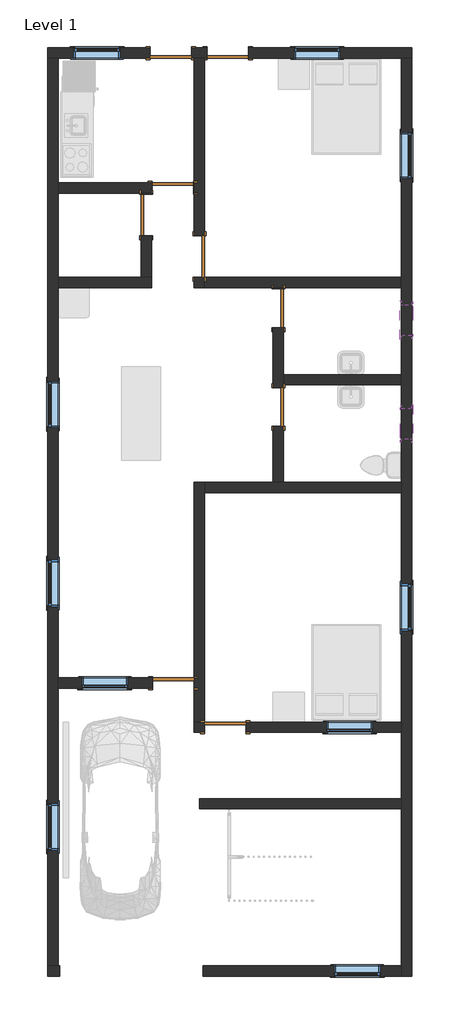
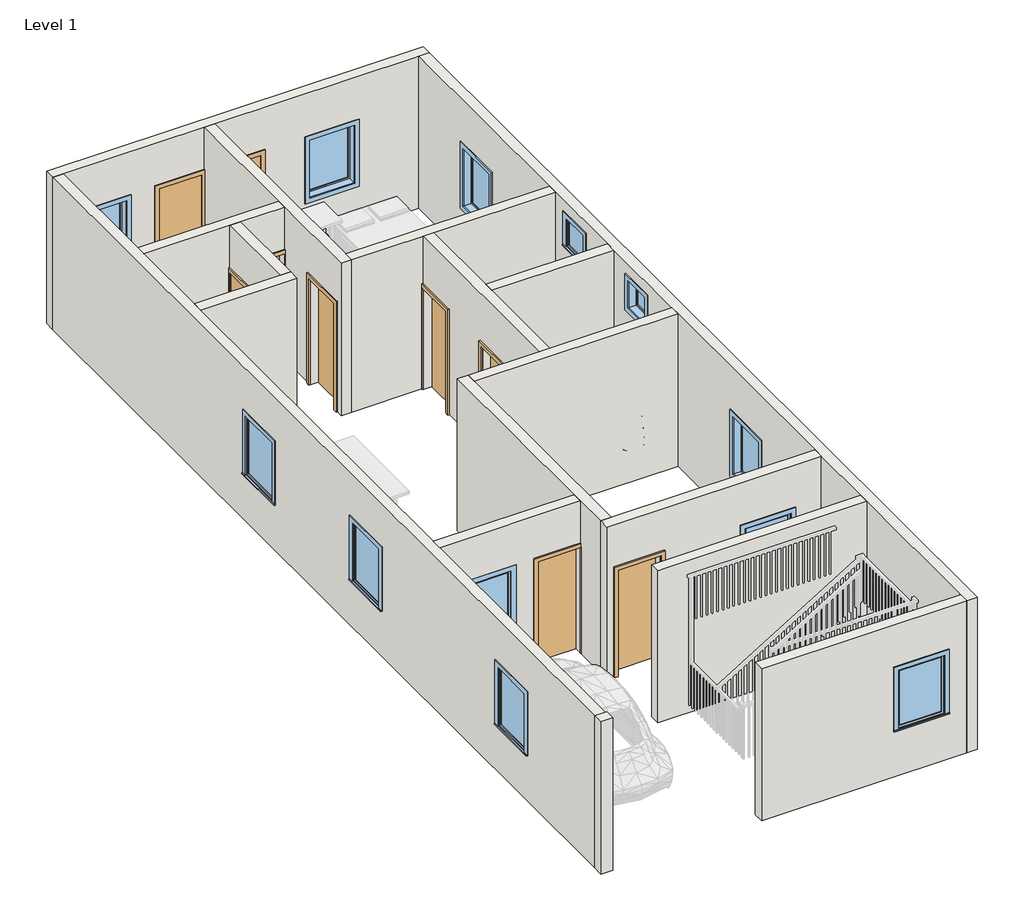
# One storey, part 1 of 3: 17 walls, 12 windows, 9 doors.
"""IFC4 building model written with IfcOpenShell, lengths in millimetres."""

from ifc_helpers import new_model, si_unit, frame, origin, origin_with_axes, place, context, project, spatial, polyline, outline, extrude, faceted_brep, transform, mapped, element, save
from components import door_53b1b562, door_64d5ae29, door_0d629d65, window_8a4441b2, window_bec2521a, window_e41d21a6

model = new_model("IFC4")

# Units and contexts
model_context = context("Model", 3, world=origin())
ifc_project = project(units=[si_unit("LENGTHUNIT", "METRE", prefix="MILLI")], contexts=[model_context])

# Site, building, storey
site = spatial("IfcSite", under=ifc_project)
building = spatial("IfcBuilding", under=site)
storey = spatial("IfcBuildingStorey", under=building, Name="Level 1", Elevation=0.0)

# Doors
placement = place(None, origin())
door_shape = door_53b1b562(model_context)
element("IfcDoor", 1, ObjectType="Single-Flush : 30\" x 80\"", at=placement, inside=storey, context=model_context, shape_type="MappedRepresentation", body=[
    mapped(door_shape, transform((-5398.5370113, 5721.2865244, 0.0), x_axis=(0.0, 1.0, 0.0), y_axis=(-1.0, 0.0, 0.0), z_axis=(0.0, 0.0, 1.0))),
])
element("IfcDoor", 2, ObjectType="Single-Flush : 30\" x 80\"", at=placement, inside=storey, context=model_context, shape_type="MappedRepresentation", body=[
    mapped(door_shape, transform((-5398.5370113, 3790.8865244, 0.0), x_axis=(0.0, 1.0, 0.0), y_axis=(-1.0, 0.0, 0.0), z_axis=(0.0, 0.0, 1.0))),
])
door_2_shape = door_64d5ae29(model_context)
element("IfcDoor", 3, ObjectType="Single-Flush : 32\" x 84\"", at=placement, inside=storey, context=model_context, shape_type="MappedRepresentation", body=[
    mapped(door_2_shape, transform((-7468.6370113, 8083.4865244, 0.0), x_axis=(1.0, 0.0, 0.0), y_axis=(0.0, 1.0, 0.0), z_axis=(0.0, 0.0, 1.0))),
])
element("IfcDoor", 4, ObjectType="Single-Flush : 32\" x 84\"", at=placement, inside=storey, context=model_context, shape_type="MappedRepresentation", body=[
    mapped(door_2_shape, transform((-7989.3370113, 7550.0865244, 0.0), x_axis=(0.0, 1.0, 0.0), y_axis=(-1.0, 0.0, 0.0), z_axis=(0.0, 0.0, 1.0))),
])
element("IfcDoor", 5, ObjectType="Single-Flush : 32\" x 84\"", at=placement, inside=storey, context=model_context, shape_type="MappedRepresentation", body=[
    mapped(door_2_shape, transform((-6947.9370113, 6737.2865244, 0.0), x_axis=(0.0, -1.0, 0.0), y_axis=(1.0, 0.0, 0.0), z_axis=(0.0, 0.0, 1.0))),
])
element("IfcDoor", 6, ObjectType="Single-Flush : 32\" x 84\"", at=placement, inside=storey, context=model_context, shape_type="MappedRepresentation", body=[
    mapped(door_2_shape, transform((-6389.1370113, 10725.0865244, 0.0), x_axis=(-1.0, 0.0, 0.0), y_axis=(0.0, -1.0, 0.0), z_axis=(0.0, 0.0, 1.0))),
])
element("IfcDoor", 7, ObjectType="Single-Flush : 32\" x 84\"", at=placement, inside=storey, context=model_context, shape_type="MappedRepresentation", body=[
    mapped(door_2_shape, transform((-7455.9370113, -1619.3134756, 0.0), x_axis=(1.0, 0.0, 0.0), y_axis=(0.0, 1.0, 0.0), z_axis=(0.0, 0.0, 1.0))),
])
door_3_shape = door_0d629d65(model_context)
element("IfcDoor", 8, ObjectType="Single-Flush : 32\" x 84\"", at=placement, inside=storey, context=model_context, shape_type="MappedRepresentation", body=[
    mapped(door_3_shape, transform((-7506.7370113, 10725.0865244, 0.0), x_axis=(1.0, 0.0, 0.0), y_axis=(0.0, 1.0, 0.0), z_axis=(0.0, 0.0, 1.0))),
])
element("IfcDoor", 9, ObjectType="Single-Flush : 32\" x 84\"", at=placement, inside=storey, context=model_context, shape_type="MappedRepresentation", body=[
    mapped(door_3_shape, transform((-6439.9370113, -2482.9134756, 0.0), x_axis=(-1.0, 0.0, 0.0), y_axis=(0.0, -1.0, 0.0), z_axis=(0.0, 0.0, 1.0))),
])

# Walls
element("IfcWall", 10, ObjectType="Generic - 8\"", at=placement, inside=storey, context=model_context, shape_type="Brep", body=[
    faceted_brep([(-7100.3370113, 10623.4865244, 0.0), (-7049.5370113, 10623.4865244, 0.0), (-6846.3370113, 10623.4865244, 0.0), (-6795.5370113, 10623.4865244, 0.0), (-6795.5370113, 10623.4865244, 2133.6), (-5982.7370113, 10623.4865244, 2133.6), (-5982.7370113, 10623.4865244, 0.0), (-2985.5370113, 10623.4865244, 0.0), (-2782.3370113, 10623.4865244, 0.0), (-2782.3370113, 10623.4865244, 3048.0), (-2985.5370113, 10623.4865244, 3048.0), (-6846.3370113, 10623.4865244, 3048.0), (-7049.5370113, 10623.4865244, 3048.0), (-9716.5370113, 10623.4865244, 3048.0), (-9919.7370113, 10623.4865244, 3048.0), (-9919.7370113, 10623.4865244, 0.0), (-9716.5370113, 10623.4865244, 0.0), (-7913.1370113, 10623.4865244, 0.0), (-7913.1370113, 10623.4865244, 2133.6), (-7100.3370113, 10623.4865244, 2133.6), (-4179.3370113, 10623.4865244, 2133.6), (-4179.3370113, 10623.4865244, 914.4), (-5093.7370113, 10623.4865244, 914.4), (-5093.7370113, 10623.4865244, 2133.6), (-8497.3370113, 10623.4865244, 2133.6), (-8497.3370113, 10623.4865244, 914.4), (-9411.7370113, 10623.4865244, 914.4), (-9411.7370113, 10623.4865244, 2133.6), (-6795.5370113, 10826.6865244, 2133.6), (-6795.5370113, 10826.6865244, 0.0), (-7100.3370113, 10826.6865244, 0.0), (-7100.3370113, 10826.6865244, 2133.6), (-7913.1370113, 10826.6865244, 2133.6), (-7913.1370113, 10826.6865244, 0.0), (-9919.7370113, 10826.6865244, 0.0), (-9919.7370113, 10826.6865244, 3048.0), (-2782.3370113, 10826.6865244, 3048.0), (-2782.3370113, 10826.6865244, 0.0), (-5982.7370113, 10826.6865244, 0.0), (-5982.7370113, 10826.6865244, 2133.6), (-4179.3370113, 10826.6865244, 2133.6), (-5093.7370113, 10826.6865244, 2133.6), (-5093.7370113, 10826.6865244, 914.4), (-4179.3370113, 10826.6865244, 914.4), (-8497.3370113, 10826.6865244, 2133.6), (-9411.7370113, 10826.6865244, 2133.6), (-9411.7370113, 10826.6865244, 914.4), (-8497.3370113, 10826.6865244, 914.4)], [[[0, 1, 2, 3, 4, 5, 6, 7, 8, 9, 10, 11, 12, 13, 14, 15, 16, 17, 18, 19], [20, 21, 22, 23], [24, 25, 26, 27]], [[28, 29, 30, 31, 32, 33, 34, 35, 36, 37, 38, 39], [40, 41, 42, 43], [44, 45, 46, 47]], [[17, 16, 15, 34, 33]], [[38, 37, 8, 7, 6]], [[30, 29, 3, 2, 1, 0]], [[14, 13, 12, 11, 10, 9, 36, 35]], [[9, 8, 37, 36]], [[15, 14, 35, 34]], [[31, 30, 0, 19]], [[32, 31, 19, 18]], [[33, 32, 18, 17]], [[4, 3, 29, 28]], [[5, 4, 28, 39]], [[6, 5, 39, 38]], [[21, 20, 40, 43]], [[22, 21, 43, 42]], [[23, 22, 42, 41]], [[20, 23, 41, 40]], [[25, 24, 44, 47]], [[26, 25, 47, 46]], [[27, 26, 46, 45]], [[24, 27, 45, 44]]]),
])
element("IfcWall", 11, ObjectType="Generic - 8\"", at=placement, inside=storey, context=model_context, shape_type="Brep", body=[
    faceted_brep([(-2985.5370113, 10623.4865244, 0.0), (-2985.5370113, 6330.8865244, 0.0), (-2985.5370113, 6127.6865244, 0.0), (-2985.5370113, 4425.8865244, 0.0), (-2985.5370113, 4222.6865244, 0.0), (-2985.5370113, 2317.6865244, 0.0), (-2985.5370113, 2114.4865244, 0.0), (-2985.5370113, -2381.3134756, 0.0), (-2985.5370113, -2584.5134756, 0.0), (-2985.5370113, -3879.9134756, 0.0), (-2985.5370113, -4083.1134756, 0.0), (-2985.5370113, -7156.5134756, 0.0), (-2985.5370113, -7359.7134756, 0.0), (-2985.5370113, -7359.7134756, 3048.0), (-2985.5370113, -7156.5134756, 3048.0), (-2985.5370113, -4083.1134756, 3048.0), (-2985.5370113, -3879.9134756, 3048.0), (-2985.5370113, -2584.5134756, 3048.0), (-2985.5370113, -2381.3134756, 3048.0), (-2985.5370113, 2114.4865244, 3048.0), (-2985.5370113, 2317.6865244, 3048.0), (-2985.5370113, 4222.6865244, 3048.0), (-2985.5370113, 4425.8865244, 3048.0), (-2985.5370113, 6127.6865244, 3048.0), (-2985.5370113, 6330.8865244, 3048.0), (-2985.5370113, 10623.4865244, 3048.0), (-2985.5370113, -590.6134756, 2133.6), (-2985.5370113, -590.6134756, 914.4), (-2985.5370113, 323.7865244, 914.4), (-2985.5370113, 323.7865244, 2133.6), (-2985.5370113, 8261.2865244, 2133.6), (-2985.5370113, 8261.2865244, 914.4), (-2985.5370113, 9175.6865244, 914.4), (-2985.5370113, 9175.6865244, 2133.6), (-2985.5370113, 5797.4865244, 2768.6), (-2985.5370113, 5187.8865244, 2768.6), (-2985.5370113, 5187.8865244, 2159.0), (-2985.5370113, 5797.4865244, 2159.0), (-2985.5370113, 3155.8865244, 2768.6), (-2985.5370113, 3155.8865244, 2159.0), (-2985.5370113, 3765.4865244, 2159.0), (-2985.5370113, 3765.4865244, 2768.6), (-2782.3370113, 10623.4865244, 0.0), (-2782.3370113, 10623.4865244, 3048.0), (-2782.3370113, -7359.7134756, 3048.0), (-2782.3370113, -7359.7134756, 0.0), (-2782.3370113, -590.6134756, 2133.6), (-2782.3370113, 323.7865244, 2133.6), (-2782.3370113, 323.7865244, 914.4), (-2782.3370113, -590.6134756, 914.4), (-2782.3370113, 8261.2865244, 2133.6), (-2782.3370113, 9175.6865244, 2133.6), (-2782.3370113, 9175.6865244, 914.4), (-2782.3370113, 8261.2865244, 914.4), (-2782.3370113, 5797.4865244, 2768.6), (-2782.3370113, 5797.4865244, 2159.0), (-2782.3370113, 5187.8865244, 2159.0), (-2782.3370113, 5187.8865244, 2768.6), (-2782.3370113, 3155.8865244, 2768.6), (-2782.3370113, 3765.4865244, 2768.6), (-2782.3370113, 3765.4865244, 2159.0), (-2782.3370113, 3155.8865244, 2159.0)], [[[0, 1, 2, 3, 4, 5, 6, 7, 8, 9, 10, 11, 12, 13, 14, 15, 16, 17, 18, 19, 20, 21, 22, 23, 24, 25], [26, 27, 28, 29], [30, 31, 32, 33], [34, 35, 36, 37], [38, 39, 40, 41]], [[42, 43, 44, 45], [46, 47, 48, 49], [50, 51, 52, 53], [54, 55, 56, 57], [58, 59, 60, 61]], [[12, 11, 10, 9, 8, 7, 6, 5, 4, 3, 2, 1, 0, 42, 45]], [[25, 24, 23, 22, 21, 20, 19, 18, 17, 16, 15, 14, 13, 44, 43]], [[0, 25, 43, 42]], [[13, 12, 45, 44]], [[27, 26, 46, 49]], [[28, 27, 49, 48]], [[29, 28, 48, 47]], [[26, 29, 47, 46]], [[31, 30, 50, 53]], [[32, 31, 53, 52]], [[33, 32, 52, 51]], [[30, 33, 51, 50]], [[55, 54, 34, 37]], [[56, 55, 37, 36]], [[57, 56, 36, 35]], [[54, 57, 35, 34]], [[39, 38, 58, 61]], [[40, 39, 61, 60]], [[41, 40, 60, 59]], [[38, 41, 59, 58]]]),
])
element("IfcWall", 12, ObjectType="Generic - 8\"", at=placement, inside=storey, context=model_context, shape_type="SweptSolid", body=[
    extrude(outline(polyline([(0.0, -2985.5370113), (3048.0, -2985.5370113), (3048.0, -6871.7370113), (0.0, -6871.7370113), (0.0, -2985.5370113)]), holes=[polyline([(2133.6, -4306.3370113), (2133.6, -3391.9370113), (914.4, -3391.9370113), (914.4, -4306.3370113), (2133.6, -4306.3370113)])]), frame((0.0, -7359.7134756, 0.0), z_axis=(0.0, 1.0, 0.0), x_axis=(0.0, 0.0, 1.0)), (0.0, 0.0, 1.0), 203.2),
])
element("IfcWall", 13, ObjectType="Generic - 8\"", at=placement, inside=storey, context=model_context, shape_type="Brep", body=[
    faceted_brep([(-9716.5370113, -7156.5134756, 0.0), (-9716.5370113, -1720.9134756, 0.0), (-9716.5370113, -1517.7134756, 0.0), (-9716.5370113, 6127.6865244, 0.0), (-9716.5370113, 6330.8865244, 0.0), (-9716.5370113, 7981.8865244, 0.0), (-9716.5370113, 8185.0865244, 0.0), (-9716.5370113, 10623.4865244, 0.0), (-9716.5370113, 10623.4865244, 3048.0), (-9716.5370113, 8185.0865244, 3048.0), (-9716.5370113, 7981.8865244, 3048.0), (-9716.5370113, 6330.8865244, 3048.0), (-9716.5370113, 6127.6865244, 3048.0), (-9716.5370113, -1517.7134756, 3048.0), (-9716.5370113, -1720.9134756, 3048.0), (-9716.5370113, -7156.5134756, 3048.0), (-9716.5370113, 4298.8865244, 2133.6), (-9716.5370113, 4298.8865244, 914.4), (-9716.5370113, 3384.4865244, 914.4), (-9716.5370113, 3384.4865244, 2133.6), (-9716.5370113, 793.6865244, 2133.6), (-9716.5370113, 793.6865244, 914.4), (-9716.5370113, -120.7134756, 914.4), (-9716.5370113, -120.7134756, 2133.6), (-9716.5370113, -3981.5134756, 2133.6), (-9716.5370113, -3981.5134756, 914.4), (-9716.5370113, -4895.9134756, 914.4), (-9716.5370113, -4895.9134756, 2133.6), (-9919.7370113, -7156.5134756, 0.0), (-9919.7370113, -7156.5134756, 3048.0), (-9919.7370113, 10623.4865244, 3048.0), (-9919.7370113, 10623.4865244, 0.0), (-9919.7370113, 4298.8865244, 2133.6), (-9919.7370113, 3384.4865244, 2133.6), (-9919.7370113, 3384.4865244, 914.4), (-9919.7370113, 4298.8865244, 914.4), (-9919.7370113, 793.6865244, 2133.6), (-9919.7370113, -120.7134756, 2133.6), (-9919.7370113, -120.7134756, 914.4), (-9919.7370113, 793.6865244, 914.4), (-9919.7370113, -3981.5134756, 2133.6), (-9919.7370113, -4895.9134756, 2133.6), (-9919.7370113, -4895.9134756, 914.4), (-9919.7370113, -3981.5134756, 914.4)], [[[0, 1, 2, 3, 4, 5, 6, 7, 8, 9, 10, 11, 12, 13, 14, 15], [16, 17, 18, 19], [20, 21, 22, 23], [24, 25, 26, 27]], [[28, 29, 30, 31], [32, 33, 34, 35], [36, 37, 38, 39], [40, 41, 42, 43]], [[7, 6, 5, 4, 3, 2, 1, 0, 28, 31]], [[15, 14, 13, 12, 11, 10, 9, 8, 30, 29]], [[8, 7, 31, 30]], [[0, 15, 29, 28]], [[17, 16, 32, 35]], [[18, 17, 35, 34]], [[19, 18, 34, 33]], [[16, 19, 33, 32]], [[21, 20, 36, 39]], [[22, 21, 39, 38]], [[23, 22, 38, 37]], [[20, 23, 37, 36]], [[25, 24, 40, 43]], [[26, 25, 43, 42]], [[27, 26, 42, 41]], [[24, 27, 41, 40]]]),
])
element("IfcWall", 14, ObjectType="Generic - 8\"", at=placement, inside=storey, context=model_context, shape_type="Brep", body=[
    faceted_brep([(-7062.2370113, 7981.8865244, 2133.6), (-7062.2370113, 7981.8865244, 0.0), (-7049.5370113, 7981.8865244, 0.0), (-7049.5370113, 7981.8865244, 3048.0), (-7887.7370113, 7981.8865244, 3048.0), (-8090.9370113, 7981.8865244, 3048.0), (-9716.5370113, 7981.8865244, 3048.0), (-9716.5370113, 7981.8865244, 0.0), (-8090.9370113, 7981.8865244, 0.0), (-7887.7370113, 7981.8865244, 0.0), (-7875.0370113, 7981.8865244, 0.0), (-7875.0370113, 7981.8865244, 2133.6), (-7049.5370113, 8185.0865244, 0.0), (-7062.2370113, 8185.0865244, 0.0), (-7062.2370113, 8185.0865244, 2133.6), (-7875.0370113, 8185.0865244, 2133.6), (-7875.0370113, 8185.0865244, 0.0), (-9716.5370113, 8185.0865244, 0.0), (-9716.5370113, 8185.0865244, 3048.0), (-7049.5370113, 8185.0865244, 3048.0)], [[[0, 1, 2, 3, 4, 5, 6, 7, 8, 9, 10, 11]], [[12, 13, 14, 15, 16, 17, 18, 19]], [[2, 1, 13, 12]], [[10, 9, 8, 7, 17, 16]], [[6, 5, 4, 3, 19, 18]], [[7, 6, 18, 17]], [[3, 2, 12, 19]], [[14, 13, 1, 0]], [[15, 14, 0, 11]], [[16, 15, 11, 10]]]),
])
element("IfcWall", 15, ObjectType="Generic - 8\"", at=placement, inside=storey, context=model_context, shape_type="Brep", body=[
    faceted_brep([(-9716.5370113, 6127.6865244, 0.0), (-7887.7370113, 6127.6865244, 0.0), (-7887.7370113, 6127.6865244, 3048.0), (-9716.5370113, 6127.6865244, 3048.0), (-9716.5370113, 6330.8865244, 0.0), (-9716.5370113, 6330.8865244, 3048.0), (-8090.9370113, 6330.8865244, 3048.0), (-7887.7370113, 6330.8865244, 3048.0), (-7887.7370113, 6330.8865244, 0.0), (-8090.9370113, 6330.8865244, 0.0)], [[[0, 1, 2, 3]], [[4, 5, 6, 7, 8, 9]], [[1, 0, 4, 9, 8]], [[3, 2, 7, 6, 5]], [[0, 3, 5, 4]], [[2, 1, 8, 7]]]),
])
element("IfcWall", 16, ObjectType="Generic - 8\"", at=placement, inside=storey, context=model_context, shape_type="SweptSolid", body=[
    extrude(outline(polyline([(7981.8865244, 0.0), (7956.4865244, 0.0), (7956.4865244, 2133.6), (7143.6865244, 2133.6), (7143.6865244, 0.0), (6330.8865244, 0.0), (6330.8865244, 3048.0), (7981.8865244, 3048.0), (7981.8865244, 0.0)])), frame((-8090.9370113, 0.0, 0.0), z_axis=(1.0, 0.0, 0.0), x_axis=(0.0, 1.0, 0.0)), (0.0, 0.0, 1.0), 203.2),
])
element("IfcWall", 17, ObjectType="Generic - 8\"", at=placement, inside=storey, context=model_context, shape_type="SweptSolid", body=[
    extrude(outline(polyline([(3048.0, -7049.5370113), (3048.0, -9716.5370113), (0.0, -9716.5370113), (0.0, -7862.3370113), (2133.6, -7862.3370113), (2133.6, -7049.5370113), (3048.0, -7049.5370113)]), holes=[polyline([(2133.6, -9259.3370113), (2133.6, -8344.9370113), (914.4, -8344.9370113), (914.4, -9259.3370113), (2133.6, -9259.3370113)])]), frame((0.0, -1720.9134756, 0.0), z_axis=(0.0, 1.0, 0.0), x_axis=(0.0, 0.0, 1.0)), (0.0, 0.0, 1.0), 203.2),
])
element("IfcWall", 18, ObjectType="Generic - 8\"", at=placement, inside=storey, context=model_context, shape_type="SweptSolid", body=[
    extrude(outline(polyline([(-6947.9370113, -3879.9134756), (-2985.5370113, -3879.9134756), (-2985.5370113, -4083.1134756), (-6947.9370113, -4083.1134756), (-6947.9370113, -3879.9134756)])), origin_with_axes(), (0.0, 0.0, 1.0), 3048.0),
])
element("IfcWall", 19, ObjectType="Generic - 8\"", at=placement, inside=storey, context=model_context, shape_type="Brep", body=[
    faceted_brep([(-6846.3370113, -2381.3134756, 2133.6), (-6846.3370113, -2381.3134756, 0.0), (-7049.5370113, -2381.3134756, 0.0), (-7049.5370113, -2381.3134756, 3048.0), (-6846.3370113, -2381.3134756, 3048.0), (-2985.5370113, -2381.3134756, 3048.0), (-2985.5370113, -2381.3134756, 0.0), (-6033.5370113, -2381.3134756, 0.0), (-6033.5370113, -2381.3134756, 2133.6), (-4458.7370113, -2381.3134756, 2133.6), (-4458.7370113, -2381.3134756, 914.4), (-3544.3370113, -2381.3134756, 914.4), (-3544.3370113, -2381.3134756, 2133.6), (-7049.5370113, -2584.5134756, 0.0), (-6846.3370113, -2584.5134756, 0.0), (-6846.3370113, -2584.5134756, 2133.6), (-6033.5370113, -2584.5134756, 2133.6), (-6033.5370113, -2584.5134756, 0.0), (-2985.5370113, -2584.5134756, 0.0), (-2985.5370113, -2584.5134756, 3048.0), (-7049.5370113, -2584.5134756, 3048.0), (-4458.7370113, -2584.5134756, 2133.6), (-3544.3370113, -2584.5134756, 2133.6), (-3544.3370113, -2584.5134756, 914.4), (-4458.7370113, -2584.5134756, 914.4)], [[[0, 1, 2, 3, 4, 5, 6, 7, 8], [9, 10, 11, 12]], [[13, 14, 15, 16, 17, 18, 19, 20], [21, 22, 23, 24]], [[7, 6, 18, 17]], [[2, 1, 14, 13]], [[5, 4, 3, 20, 19]], [[6, 5, 19, 18]], [[15, 14, 1, 0]], [[16, 15, 0, 8]], [[17, 16, 8, 7]], [[3, 2, 13, 20]], [[10, 9, 21, 24]], [[11, 10, 24, 23]], [[12, 11, 23, 22]], [[9, 12, 22, 21]]]),
])
element("IfcWall", 20, ObjectType="Generic - 8\"", at=placement, inside=storey, context=model_context, shape_type="Brep", body=[
    faceted_brep([(-2985.5370113, 2317.6865244, 0.0), (-5296.9370113, 2317.6865244, 0.0), (-5500.1370113, 2317.6865244, 0.0), (-6846.3370113, 2317.6865244, 0.0), (-6846.3370113, 2317.6865244, 3048.0), (-5500.1370113, 2317.6865244, 3048.0), (-5296.9370113, 2317.6865244, 3048.0), (-2985.5370113, 2317.6865244, 3048.0), (-2985.5370113, 2114.4865244, 0.0), (-2985.5370113, 2114.4865244, 3048.0), (-6846.3370113, 2114.4865244, 3048.0), (-6846.3370113, 2114.4865244, 0.0)], [[[0, 1, 2, 3, 4, 5, 6, 7]], [[8, 9, 10, 11]], [[3, 2, 1, 0, 8, 11]], [[7, 6, 5, 4, 10, 9]], [[0, 7, 9, 8]], [[4, 3, 11, 10]]]),
])
element("IfcWall", 21, ObjectType="Generic - 8\"", at=placement, inside=storey, context=model_context, shape_type="Brep", body=[
    faceted_brep([(-6846.3370113, 6127.6865244, 0.0), (-5500.1370113, 6127.6865244, 0.0), (-5296.9370113, 6127.6865244, 0.0), (-2985.5370113, 6127.6865244, 0.0), (-2985.5370113, 6127.6865244, 3048.0), (-5296.9370113, 6127.6865244, 3048.0), (-5500.1370113, 6127.6865244, 3048.0), (-6846.3370113, 6127.6865244, 3048.0), (-6846.3370113, 6330.8865244, 0.0), (-6846.3370113, 6330.8865244, 3048.0), (-2985.5370113, 6330.8865244, 3048.0), (-2985.5370113, 6330.8865244, 0.0)], [[[0, 1, 2, 3, 4, 5, 6, 7]], [[8, 9, 10, 11]], [[3, 2, 1, 0, 8, 11]], [[7, 6, 5, 4, 10, 9]], [[4, 3, 11, 10]], [[0, 7, 9, 8]]]),
])
element("IfcWall", 22, ObjectType="Generic - 8\"", at=placement, inside=storey, context=model_context, shape_type="SweptSolid", body=[
    extrude(outline(polyline([(-5296.9370113, 4425.8865244), (-2985.5370113, 4425.8865244), (-2985.5370113, 4222.6865244), (-5296.9370113, 4222.6865244), (-5296.9370113, 4425.8865244)])), origin_with_axes(), (0.0, 0.0, 1.0), 3048.0),
])
element("IfcWall", 23, ObjectType="Generic - 8\"", at=placement, inside=storey, context=model_context, shape_type="Brep", body=[
    faceted_brep([(-5500.1370113, 5340.2865244, 0.0), (-5500.1370113, 4171.8865244, 0.0), (-5500.1370113, 4171.8865244, 2032.0), (-5500.1370113, 3409.8865244, 2032.0), (-5500.1370113, 3409.8865244, 0.0), (-5500.1370113, 2317.6865244, 0.0), (-5500.1370113, 2317.6865244, 3048.0), (-5500.1370113, 6127.6865244, 3048.0), (-5500.1370113, 6127.6865244, 0.0), (-5500.1370113, 6102.2865244, 0.0), (-5500.1370113, 6102.2865244, 2032.0), (-5500.1370113, 5340.2865244, 2032.0), (-5296.9370113, 4171.8865244, 2032.0), (-5296.9370113, 4171.8865244, 0.0), (-5296.9370113, 4222.6865244, 0.0), (-5296.9370113, 4425.8865244, 0.0), (-5296.9370113, 5340.2865244, 0.0), (-5296.9370113, 5340.2865244, 2032.0), (-5296.9370113, 6102.2865244, 2032.0), (-5296.9370113, 6102.2865244, 0.0), (-5296.9370113, 6127.6865244, 0.0), (-5296.9370113, 6127.6865244, 3048.0), (-5296.9370113, 4425.8865244, 3048.0), (-5296.9370113, 4222.6865244, 3048.0), (-5296.9370113, 2317.6865244, 3048.0), (-5296.9370113, 2317.6865244, 0.0), (-5296.9370113, 3409.8865244, 0.0), (-5296.9370113, 3409.8865244, 2032.0)], [[[0, 1, 2, 3, 4, 5, 6, 7, 8, 9, 10, 11]], [[12, 13, 14, 15, 16, 17, 18, 19, 20, 21, 22, 23, 24, 25, 26, 27]], [[20, 19, 9, 8]], [[26, 25, 5, 4]], [[16, 15, 14, 13, 1, 0]], [[7, 6, 24, 23, 22, 21]], [[6, 5, 25, 24]], [[8, 7, 21, 20]], [[10, 9, 19, 18]], [[11, 10, 18, 17]], [[0, 11, 17, 16]], [[2, 1, 13, 12]], [[3, 2, 12, 27]], [[4, 3, 27, 26]]]),
])
element("IfcWall", 24, ObjectType="Generic - 8\"", at=placement, inside=storey, context=model_context, shape_type="Brep", body=[
    faceted_brep([(-6846.3370113, 6127.6865244, 0.0), (-6846.3370113, 6330.8865244, 0.0), (-6846.3370113, 6330.8865244, 2133.6), (-6846.3370113, 7143.6865244, 2133.6), (-6846.3370113, 7143.6865244, 0.0), (-6846.3370113, 10623.4865244, 0.0), (-6846.3370113, 10623.4865244, 3048.0), (-6846.3370113, 6330.8865244, 3048.0), (-6846.3370113, 6127.6865244, 3048.0), (-7049.5370113, 6330.8865244, 2133.6), (-7049.5370113, 6330.8865244, 0.0), (-7049.5370113, 6127.6865244, 0.0), (-7049.5370113, 6127.6865244, 3048.0), (-7049.5370113, 7981.8865244, 3048.0), (-7049.5370113, 8185.0865244, 3048.0), (-7049.5370113, 10623.4865244, 3048.0), (-7049.5370113, 10623.4865244, 0.0), (-7049.5370113, 8185.0865244, 0.0), (-7049.5370113, 7981.8865244, 0.0), (-7049.5370113, 7143.6865244, 0.0), (-7049.5370113, 7143.6865244, 2133.6)], [[[0, 1, 2, 3, 4, 5, 6, 7, 8]], [[9, 10, 11, 12, 13, 14, 15, 16, 17, 18, 19, 20]], [[11, 10, 1, 0]], [[19, 18, 17, 16, 5, 4]], [[8, 7, 6, 15, 14, 13, 12]], [[6, 5, 16, 15]], [[0, 8, 12, 11]], [[2, 1, 10, 9]], [[3, 2, 9, 20]], [[4, 3, 20, 19]]]),
])
element("IfcWall", 25, ObjectType="Generic - 8\"", at=placement, inside=storey, context=model_context, shape_type="Brep", body=[
    faceted_brep([(-6846.3370113, -2381.3134756, 0.0), (-6846.3370113, 2114.4865244, 0.0), (-6846.3370113, 2317.6865244, 0.0), (-6846.3370113, 2317.6865244, 3048.0), (-6846.3370113, 2114.4865244, 3048.0), (-6846.3370113, -2381.3134756, 3048.0), (-6846.3370113, -2381.3134756, 2133.6), (-7049.5370113, -2381.3134756, 0.0), (-7049.5370113, -2381.3134756, 3048.0), (-7049.5370113, -1720.9134756, 3048.0), (-7049.5370113, -1517.7134756, 3048.0), (-7049.5370113, 2317.6865244, 3048.0), (-7049.5370113, 2317.6865244, 0.0)], [[[0, 1, 2, 3, 4, 5, 6]], [[7, 8, 9, 10, 11, 12]], [[2, 1, 0, 7, 12]], [[5, 4, 3, 11, 10, 9, 8]], [[3, 2, 12, 11]], [[0, 6, 5, 8, 7]]]),
])
element("IfcWall", 26, ObjectType="Generic - 8\"", at=placement, inside=storey, context=model_context, shape_type="Brep", body=[
    faceted_brep([(-9691.1370113, -7156.5134756, 0.0), (-9716.5370113, -7156.5134756, 0.0), (-9919.7370113, -7156.5134756, 0.0), (-9919.7370113, -7156.5134756, 3048.0), (-9716.5370113, -7156.5134756, 3048.0), (-9691.1370113, -7156.5134756, 3048.0), (-9691.1370113, -7359.7134756, 0.0), (-9691.1370113, -7359.7134756, 3048.0), (-9919.7370113, -7359.7134756, 3048.0), (-9919.7370113, -7359.7134756, 0.0)], [[[0, 1, 2, 3, 4, 5]], [[6, 7, 8, 9]], [[2, 1, 0, 6, 9]], [[5, 4, 3, 8, 7]], [[0, 5, 7, 6]], [[3, 2, 9, 8]]]),
])

# Windows
window_shape = window_8a4441b2(model_context)
element("IfcWindow", 27, ObjectType="Casement with Trim : 36\" x 48\"", at=placement, inside=storey, context=model_context, shape_type="MappedRepresentation", body=[
    mapped(window_shape, transform((-4001.5370113, -2482.9134756, 0.0), x_axis=(-1.0, 0.0, 0.0), y_axis=(0.0, -1.0, 0.0), z_axis=(0.0, 0.0, 1.0))),
])
window_2_shape = window_bec2521a(model_context)
element("IfcWindow", 28, ObjectType="Fixed with Trim : 36\" x 48\"", at=placement, inside=storey, context=model_context, shape_type="MappedRepresentation", body=[
    mapped(window_2_shape, transform((-3887.2370113, -7258.1134756, 0.0), x_axis=(-1.0, 0.0, 0.0), y_axis=(0.0, -1.0, 0.0), z_axis=(0.0, 0.0, 1.0))),
])
element("IfcWindow", 29, ObjectType="Fixed with Trim : 36\" x 48\"", at=placement, inside=storey, context=model_context, shape_type="MappedRepresentation", body=[
    mapped(window_2_shape, transform((-2883.9370113, -171.5134756, 0.0), x_axis=(0.0, -1.0, 0.0), y_axis=(1.0, 0.0, 0.0), z_axis=(0.0, 0.0, 1.0))),
])
element("IfcWindow", 30, ObjectType="Fixed with Trim : 36\" x 48\"", at=placement, inside=storey, context=model_context, shape_type="MappedRepresentation", body=[
    mapped(window_2_shape, transform((-2883.9370113, 8680.3865244, 0.0), x_axis=(0.0, -1.0, 0.0), y_axis=(1.0, 0.0, 0.0), z_axis=(0.0, 0.0, 1.0))),
])
element("IfcWindow", 31, ObjectType="Fixed with Trim : 36\" x 48\"", at=placement, inside=storey, context=model_context, shape_type="MappedRepresentation", body=[
    mapped(window_2_shape, transform((-4598.4370113, 10725.0865244, 0.0), x_axis=(1.0, 0.0, 0.0), y_axis=(0.0, 1.0, 0.0), z_axis=(0.0, 0.0, 1.0))),
])
element("IfcWindow", 32, ObjectType="Fixed with Trim : 36\" x 48\"", at=placement, inside=storey, context=model_context, shape_type="MappedRepresentation", body=[
    mapped(window_2_shape, transform((-8916.4370113, 10725.0865244, 0.0), x_axis=(1.0, 0.0, 0.0), y_axis=(0.0, 1.0, 0.0), z_axis=(0.0, 0.0, 1.0))),
])
element("IfcWindow", 33, ObjectType="Fixed with Trim : 36\" x 48\"", at=placement, inside=storey, context=model_context, shape_type="MappedRepresentation", body=[
    mapped(window_2_shape, transform((-9818.1370113, 3879.7865244, 0.0), x_axis=(0.0, 1.0, 0.0), y_axis=(-1.0, 0.0, 0.0), z_axis=(0.0, 0.0, 1.0))),
])
element("IfcWindow", 34, ObjectType="Fixed with Trim : 36\" x 48\"", at=placement, inside=storey, context=model_context, shape_type="MappedRepresentation", body=[
    mapped(window_2_shape, transform((-9818.1370113, 374.5865244, 0.0), x_axis=(0.0, 1.0, 0.0), y_axis=(-1.0, 0.0, 0.0), z_axis=(0.0, 0.0, 1.0))),
])
element("IfcWindow", 35, ObjectType="Fixed with Trim : 36\" x 48\"", at=placement, inside=storey, context=model_context, shape_type="MappedRepresentation", body=[
    mapped(window_2_shape, transform((-9818.1370113, -4400.6134756, 0.0), x_axis=(0.0, 1.0, 0.0), y_axis=(-1.0, 0.0, 0.0), z_axis=(0.0, 0.0, 1.0))),
])
element("IfcWindow", 36, ObjectType="Fixed with Trim : 36\" x 48\"", at=placement, inside=storey, context=model_context, shape_type="MappedRepresentation", body=[
    mapped(window_2_shape, transform((-8840.2370113, -1619.3134756, 0.0), x_axis=(-1.0, 0.0, 0.0), y_axis=(0.0, -1.0, 0.0), z_axis=(0.0, 0.0, 1.0))),
])
window_3_shape = window_e41d21a6(model_context)
element("IfcWindow", 37, ObjectType="Transom with Trim : 24\" x 24\"", at=placement, inside=storey, context=model_context, shape_type="MappedRepresentation", body=[
    mapped(window_3_shape, transform((-2883.9370113, 5530.7865244, 0.0), x_axis=(0.0, 1.0, 0.0), y_axis=(-1.0, 0.0, 0.0), z_axis=(0.0, 0.0, 1.0))),
])
element("IfcWindow", 38, ObjectType="Transom with Trim : 24\" x 24\"", at=placement, inside=storey, context=model_context, shape_type="MappedRepresentation", body=[
    mapped(window_3_shape, transform((-2883.9370113, 3422.5865244, 0.0), x_axis=(0.0, -1.0, 0.0), y_axis=(1.0, 0.0, 0.0), z_axis=(0.0, 0.0, 1.0))),
])

save(model, "model.ifc")

# Revit data of these elements
# Type "Single-Flush : 30\" x 80\""
#   Type Mark = "5"
#   Construction Type Id = "MDOOR"
#   Assembly Code = "C1020"
#   Analytic Construction = "Metal"
#   Thickness = 0' - 2"
#   Heat Transfer Coefficient (U) = 0.651978 BTU/(h·ft²·°F)
#   Height = 6' - 8"
#   Trim Projection Ext = 0' - 1"
#   Trim Projection Int = 0' - 1"
#   Trim Width = 0' - 3"
#   Width = 2' - 6"
#   Define Thermal Properties by = 1
#   Door Material = Door - Panel
#   Frame Material = Door - Frame
#   Visual Light Transmittance = 0
#   Solar Heat Gain Coefficient = 0
#   Function = (empty or 0)
#   Wall Closure = (empty or 0)
# Type "Single-Flush : 32\" x 84\""
#   Type Mark = "3"
#   Construction Type Id = "MDOOR"
#   Assembly Code = "C1020"
#   Analytic Construction = "Metal"
#   Thickness = 0' - 2"
#   Heat Transfer Coefficient (U) = 0.651978 BTU/(h·ft²·°F)
#   Height = 7' - 0"
#   Trim Projection Ext = 0' - 1"
#   Trim Projection Int = 0' - 1"
#   Trim Width = 0' - 3"
#   Width = 2' - 8"
#   Define Thermal Properties by = 1
#   Door Material = Door - Panel
#   Frame Material = Door - Frame
#   Visual Light Transmittance = 0
#   Solar Heat Gain Coefficient = 0
#   Function = (empty or 0)
#   Wall Closure = (empty or 0)
# Type "Generic - 8\""
#   Assembly Code = "B2010"
#   Layers, outside or top first: 0' - 8" no material (function 1)
# Type "Casement with Trim : 36\" x 48\""
#   Type Mark = "29"
#   Construction Type Id = "GSP4R"
#   Assembly Code = "B2020100"
#   Analytic Construction = "1/8 in Pilkington single glazing"
#   Visual Light Transmittance = 0.9
#   Solar Heat Gain Coefficient = 0.78
#   Heat Transfer Coefficient (U) = 0.6496 BTU/(h·ft²·°F)
#   Height = 4' - 0"
#   Default Sill Height = 3' - 0"
#   Trim Projection - Ext. = 0' - 0 1/2"
#   Trim Projection - Int. = 0' - 0 3/4"
#   Trim Width - Exterior = 0' - 3 1/2"
#   Trim Width - Interior = 0' - 3 1/2"
#   Width = 3' - 0"
#   Window Inset = 0' - 0 3/4"
#   Define Thermal Properties by = 1
#   Glass Pane Material = Glass
#   Sash Material = Sash
#   Trim Exterior Material = Trim
#   Trim Interior Material = Trim
#   Wall Closure = (empty or 0)
# Type "Fixed with Trim : 36\" x 48\""
#   Type Mark = "10"
#   Construction Type Id = "GSP4R"
#   Assembly Code = "B2020100"
#   Analytic Construction = "1/8 in Pilkington single glazing"
#   Visual Light Transmittance = 0.9
#   Solar Heat Gain Coefficient = 0.78
#   Heat Transfer Coefficient (U) = 0.6496 BTU/(h·ft²·°F)
#   Height = 4' - 0"
#   Default Sill Height = 3' - 0"
#   Trim Projection - Ext. = 0' - 0 1/2"
#   Trim Projection - Int. = 0' - 0 3/4"
#   Trim Width - Exterior = 0' - 3 1/2"
#   Trim Width - Interior = 0' - 3 1/2"
#   Width = 3' - 0"
#   Window Inset = 0' - 0 3/4"
#   Define Thermal Properties by = 1
#   Glass Pane Material = Glass
#   Sash Material = Sash
#   Trim Exterior Material = Trim
#   Trim Interior Material = Trim
#   Wall Closure = (empty or 0)
# Type "Transom with Trim : 24\" x 24\""
#   Type Mark = "19"
#   Construction Type Id = "GSP4R"
#   Assembly Code = "B2020100"
#   Analytic Construction = "1/8 in Pilkington single glazing"
#   Visual Light Transmittance = 0.9
#   Solar Heat Gain Coefficient = 0.78
#   Heat Transfer Coefficient (U) = 0.6496 BTU/(h·ft²·°F)
#   Height = 2' - 0"
#   Default Sill Height = 7' - 1"
#   Trim Projection - Ext. = 0' - 0 1/2"
#   Trim Projection - Int. = 0' - 0 3/4"
#   Trim Width - Exterior = 0' - 3 1/2"
#   Trim Width - Interior = 0' - 3 1/2"
#   Width = 2' - 0"
#   Window Inset = 0' - 0 3/4"
#   Define Thermal Properties by = 1
#   Glass Pane Material = Glass
#   Sash Material = Sash
#   Trim Exterior Material = Trim
#   Trim Interior Material = Trim
#   Wall Closure = (empty or 0)
# Elements 1, 2 (IfcDoor, "Single-Flush : 30\" x 80\"")
#   Phase Created = New Construction
#   Materials on its faces: "Door - Frame", "Door - Panel"
# Elements 3, 4, 5, 6, 7, 8, 9 (IfcDoor, "Single-Flush : 32\" x 84\"")
#   Phase Created = New Construction
#   Materials on its faces: "Door - Frame", "Door - Panel"
# Elements 10, 11, 12, 13, 14, 15, 16, 17, 18, 19, 20, 21, 22, 23, 24, 25, 26 (IfcWall, "Generic - 8\"")
#   Top Offset = 0' - 0"
#   Base Offset = 0' - 0"
#   Unconnected Height = 10' - 0"
#   wall height = 10' - 0"
#   Phase Created = New Construction
#   Base Constraint = Level 1
#   Materials on its faces: "Default Wall"
# Element 27 (IfcWindow, "Casement with Trim : 36\" x 48\"")
#   Mark = "13"
#   Phase Created = New Construction
#   Materials on its faces: "Sash", "Trim", "Glass"
# Element 28 (IfcWindow, "Fixed with Trim : 36\" x 48\"")
#   Mark = "1"
#   Phase Created = New Construction
#   Materials on its faces: "Sash", "Trim", "Glass"
# Element 29 (IfcWindow, "Fixed with Trim : 36\" x 48\"")
#   Mark = "2"
#   Phase Created = New Construction
#   Materials on its faces: "Sash", "Trim", "Glass"
# Element 30 (IfcWindow, "Fixed with Trim : 36\" x 48\"")
#   Mark = "3"
#   Phase Created = New Construction
#   Materials on its faces: "Sash", "Trim", "Glass"
# Element 31 (IfcWindow, "Fixed with Trim : 36\" x 48\"")
#   Mark = "4"
#   Phase Created = New Construction
#   Materials on its faces: "Sash", "Trim", "Glass"
# Element 32 (IfcWindow, "Fixed with Trim : 36\" x 48\"")
#   Mark = "5"
#   Phase Created = New Construction
#   Materials on its faces: "Sash", "Trim", "Glass"
# Element 33 (IfcWindow, "Fixed with Trim : 36\" x 48\"")
#   Mark = "6"
#   Phase Created = New Construction
#   Materials on its faces: "Sash", "Trim", "Glass"
# Element 34 (IfcWindow, "Fixed with Trim : 36\" x 48\"")
#   Mark = "7"
#   Phase Created = New Construction
#   Materials on its faces: "Sash", "Trim", "Glass"
# Element 35 (IfcWindow, "Fixed with Trim : 36\" x 48\"")
#   Mark = "8"
#   Phase Created = New Construction
#   Materials on its faces: "Sash", "Trim", "Glass"
# Element 36 (IfcWindow, "Fixed with Trim : 36\" x 48\"")
#   Mark = "9"
#   Phase Created = New Construction
#   Materials on its faces: "Sash", "Trim", "Glass"
# Element 37 (IfcWindow, "Transom with Trim : 24\" x 24\"")
#   Mark = "10"
#   Phase Created = New Construction
#   Materials on its faces: "Sash", "Trim", "Glass"
# Element 38 (IfcWindow, "Transom with Trim : 24\" x 24\"")
#   Mark = "11"
#   Phase Created = New Construction
#   Materials on its faces: "Sash", "Trim", "Glass"
# Materials
#   "Door - Panel": class "Wood", colour RGB 210 159 95, transparency 0
#   "Door - Frame": colour RGB 118 70 51, transparency 0
#   "Glass": class "Glass", colour RGB 0 128 192, transparency 0.75, Description = "Soda Lime Glass", Cost = 0
#   "Sash": class "Wood", colour RGB 224 178 126, transparency 0
#   "Trim": class "Wood", colour RGB 224 178 126, transparency 0
#   "Default Wall": colour RGB 128 128 128, transparency 0
# Room at (-8240.091, 9547.878) mm, phase "New Construction", upper level "Level 1", upper offset 10' - 0", lower offset 0' - 0"
#   Number = "AREA"
#   Name = "KITCHEN"
# Room at (-8977.887, 7326.911) mm, phase "New Construction", upper level "Level 1", upper offset 10' - 0", lower offset 0' - 0"
#   Number = "ROOM"
#   Name = "STORE"
# Room at (-8240.091, 2525.649) mm, phase "New Construction", upper level "Level 1", upper offset 10' - 0", lower offset 0' - 0"
#   Number = "AREA"
#   Name = "DRAWING"
# Room at (-8493.953, -3751.214) mm, phase "New Construction", upper level "Level 1", upper offset 10' - 0", lower offset 0' - 0"
#   Number = "AREA"
#   Name = "PARKING"
# Room at (-5027.081, 682.733) mm, phase "New Construction", upper level "Level 1", upper offset 10' - 0", lower offset 0' - 0"
#   Number = "2"
#   Name = "BED ROOM"
# Room at (-4096.499, 3474.478) mm, phase "New Construction", upper level "Level 1", upper offset 10' - 0", lower offset 0' - 0"
#   Number = "ROOM"
#   Name = "WC"
# Room at (-4096.499, 5737.068) mm, phase "New Construction", upper level "Level 1", upper offset 10' - 0", lower offset 0' - 0"
#   Number = "ROOM"
#   Name = "BATH"
# Room at (-5027.081, 8589.066) mm, phase "New Construction", upper level "Level 1", upper offset 10' - 0", lower offset 0' - 0"
#   Number = "1"
#   Name = "BED ROOM"
